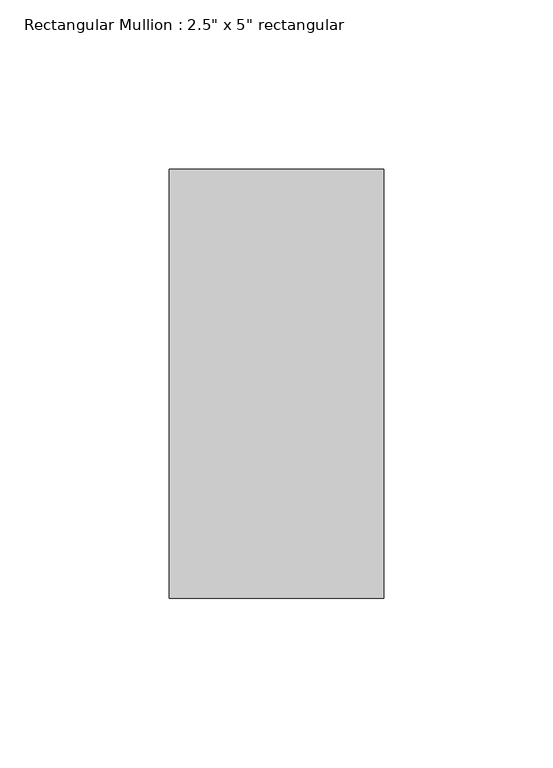
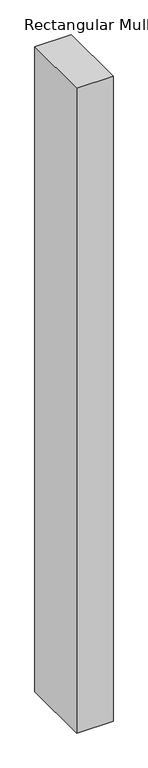
"""IFC4 building model written with IfcOpenShell, lengths in millimetres: member geometry."""

from ifc_helpers import new_model, si_unit, frame, origin, place, context, project, spatial, polyline, outline, extrude, source, transform, mapped, element, save


def member_83167d3d(model_context):
    return source(origin(), model_context, "Body", "SweptSolid", [
        extrude(outline(polyline([(0.0, 63.5), (0.0, -63.5), (-63.5, -63.5), (-63.5, 63.5), (0.0, 63.5)])), frame((0.0, 0.0, -1193.8), z_axis=(0.0, 0.0, 1.0), x_axis=(1.0, 0.0, 0.0)), (0.0, 0.0, 1.0), 1193.8),
    ])


if __name__ == "__main__":
    model = new_model("IFC4")
    model_context = context("Model", 3, world=origin())
    ifc_project = project(units=[si_unit("LENGTHUNIT", "METRE", prefix="MILLI")], contexts=[model_context])
    site = spatial("IfcSite", under=ifc_project)
    building = spatial("IfcBuilding", under=site)
    placement = place(None, origin())
    member_shape = member_83167d3d(model_context)
    element("IfcMember", 1, ObjectType="Rectangular Mullion : 2.5\" x 5\" rectangular", at=placement, inside=building, context=model_context, shape_type="MappedRepresentation", body=[
        mapped(member_shape, transform((0.0, 0.0, 0.0), x_axis=(1.0, 0.0, 0.0), y_axis=(0.0, 1.0, 0.0), z_axis=(0.0, 0.0, 1.0))),
    ])
    save(model, "model.ifc")

# Revit data of these elements
# Type "Rectangular Mullion : 2.5\" x 5\" rectangular"
#   built-in parameter 1007304 = 0.416667 (stored number, unit not read)
#   built-in parameter 1007301 = 0.104167 (stored number, unit not read)
#   built-in parameter 1007300 = 0.104167 (stored number, unit not read)
